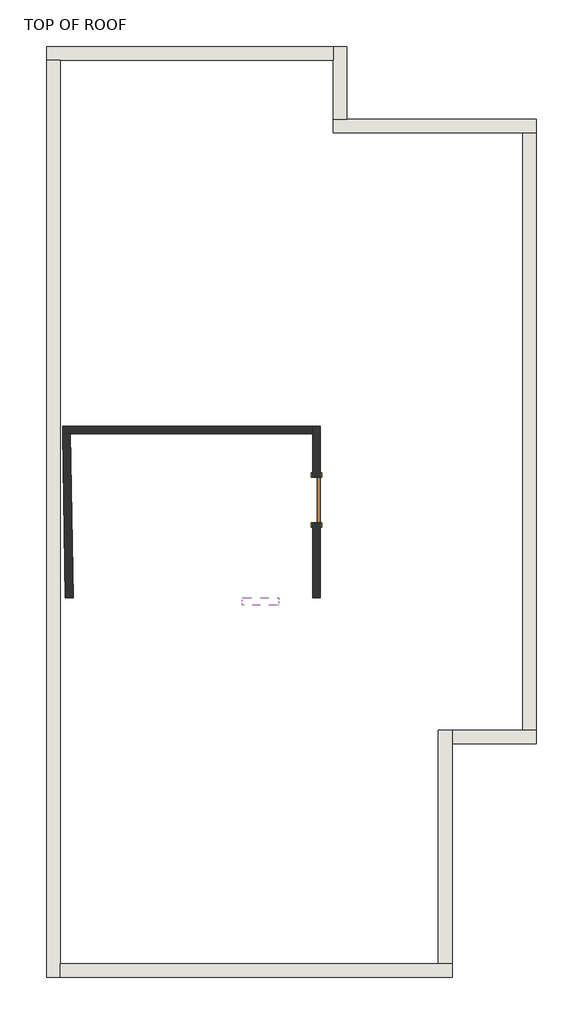
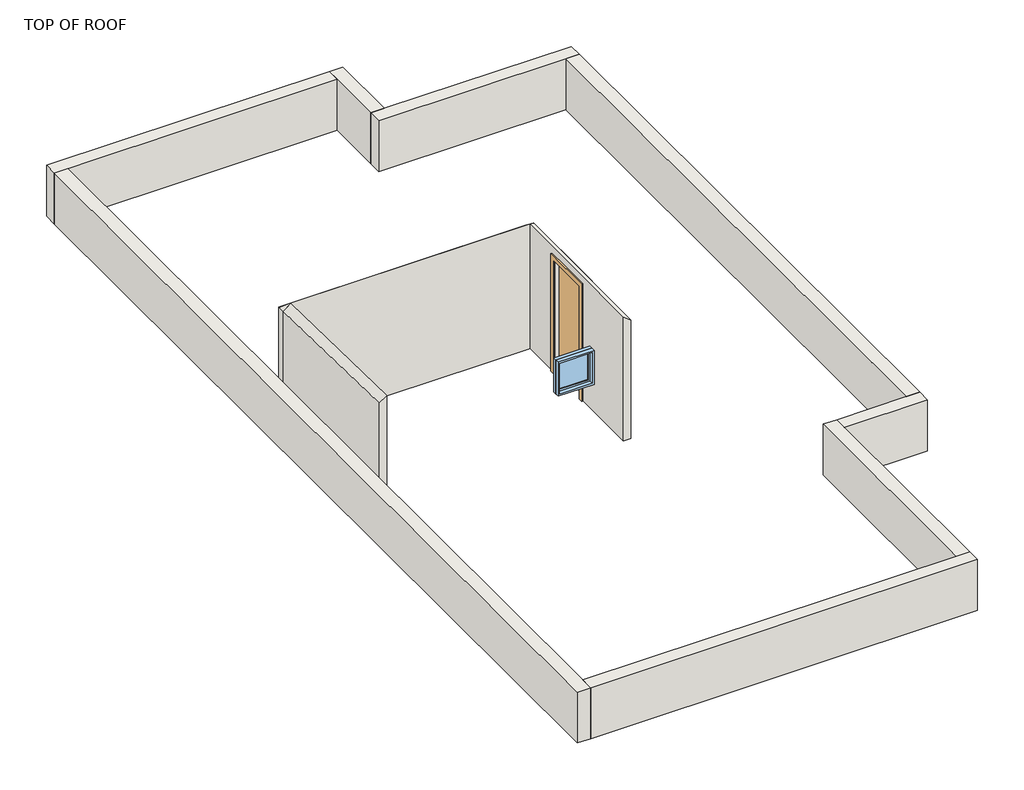
# One storey, incomplete: 11 walls, 1 door, 1 window.
"""IFC4 building model written with IfcOpenShell, lengths in millimetres."""

from ifc_helpers import new_model, si_unit, frame, origin, place, context, project, spatial, polyline, outline, extrude, faceted_brep, transform, mapped, element, save
from components import door_1fe7f57d, window_d757e824

model = new_model("IFC4")

# Units and contexts
model_context = context("Model", 3, world=origin())
ifc_project = project(units=[si_unit("LENGTHUNIT", "METRE", prefix="MILLI")], contexts=[model_context])

# Site, building, storey
site = spatial("IfcSite", under=ifc_project)
building = spatial("IfcBuilding", under=site)
storey = spatial("IfcBuildingStorey", under=building, Name="TOP OF ROOF", Elevation=6400.8)

# Door
placement = place(None, origin())
door_shape = door_1fe7f57d(model_context)
element("IfcDoor", 1, ObjectType="Single-Flush : 30\" x 80\"", at=placement, inside=storey, context=model_context, shape_type="MappedRepresentation", body=[
    mapped(door_shape, transform((-2786.5718918, 4228.995896, 6400.8), x_axis=(0.0, -1.0, 0.0), y_axis=(1.0, 0.0, 0.0), z_axis=(0.0, 0.0, 1.0))),
])

# Walls
element("IfcWall", 2, ObjectType="INNER WALL 5\"", at=placement, inside=storey, context=model_context, shape_type="Brep", body=[
    faceted_brep([(-2723.0718918, 2590.695896, 6400.8), (-2723.0718918, 3847.995896, 6400.8), (-2723.0718918, 3847.995896, 8432.8), (-2723.0718918, 4609.995896, 8432.8), (-2723.0718918, 4609.995896, 6400.8), (-2723.0718918, 5460.895896, 6400.8), (-2723.0718918, 5460.895896, 8534.4), (-2723.0718918, 5449.6118978, 8534.4), (-2723.0718918, 2590.695896, 8534.4), (-2850.0718918, 3847.995896, 8432.8), (-2850.0718918, 3847.995896, 6400.8), (-2850.0718918, 2590.695896, 6400.8), (-2850.0718918, 2590.695896, 8629.65), (-2850.0718918, 5333.895896, 8629.65), (-2850.0718918, 5337.666737, 8629.65), (-2850.0718918, 5449.6118978, 8534.4), (-2850.0718918, 5460.895896, 8534.4), (-2850.0718918, 5460.895896, 6400.8), (-2850.0718918, 5333.895896, 6400.8), (-2850.0718918, 4609.995896, 6400.8), (-2850.0718918, 4609.995896, 8432.8)], [[[0, 1, 2, 3, 4, 5, 6, 7, 8]], [[9, 10, 11, 12, 13, 14, 15, 16, 17, 18, 19, 20]], [[11, 10, 1, 0]], [[19, 18, 17, 5, 4]], [[0, 8, 12, 11]], [[6, 5, 17, 16]], [[8, 7, 14, 13, 12]], [[7, 6, 16, 15]], [[15, 14, 7]], [[2, 1, 10, 9]], [[3, 2, 9, 20]], [[4, 3, 20, 19]]]),
])
element("IfcWall", 3, ObjectType="INNER WALL 5\"", at=placement, inside=storey, context=model_context, shape_type="Brep", body=[
    faceted_brep([(-2850.0718918, 5460.895896, 6400.8), (-7041.0718918, 5460.895896, 6400.8), (-7041.0718918, 5460.895896, 8534.4), (-2850.0718918, 5460.895896, 8534.4), (-2850.0718918, 5333.895896, 6400.8), (-2850.0718918, 5333.895896, 8629.65), (-2854.3498507, 5333.895896, 8632.8584692), (-6907.6225354, 5333.895896, 8632.8584692), (-6911.9011088, 5333.895896, 8629.65), (-7038.9193494, 5333.895896, 8534.4), (-7038.9193494, 5333.895896, 6400.8), (-6911.9011088, 5333.895896, 6400.8), (-2850.0718918, 5449.6118978, 8534.4), (-2850.0718918, 5337.666737, 8629.65), (-7040.8806375, 5449.6118978, 8534.4)], [[[0, 1, 2, 3]], [[4, 5, 6, 7, 8, 9, 10, 11]], [[1, 0, 4, 11, 10]], [[0, 3, 12, 13, 5, 4]], [[2, 1, 10, 9, 14]], [[3, 2, 14, 12]], [[14, 9, 8, 7]], [[7, 6, 13, 12, 14]], [[6, 5, 13]]]),
])
element("IfcWall", 4, ObjectType="INNER WALL 5\"", at=placement, inside=storey, context=model_context, shape_type="Brep", body=[
    faceted_brep([(-7038.9193494, 5333.895896, 6400.8), (-6992.4244341, 2590.695896, 6400.8), (-6992.4244341, 2590.695896, 8534.4), (-7038.9193494, 5333.895896, 8534.4), (-6911.9011088, 5333.895896, 6400.8), (-6911.9011088, 5333.895896, 8629.65), (-6865.4061936, 2590.695896, 8629.65), (-6865.4061936, 2590.695896, 6400.8)], [[[0, 1, 2, 3]], [[4, 5, 6, 7]], [[1, 0, 4, 7]], [[2, 1, 7, 6]], [[0, 3, 5, 4]], [[3, 2, 6, 5]]]),
])
element("IfcWall", 5, ObjectType="OUTER WALL 9\"", at=placement, inside=storey, context=model_context, shape_type="Brep", body=[
    faceted_brep([(895.326752, 10603.9133697, 6400.8), (-2279.673248, 10603.9133697, 6400.8), (-2508.273248, 10603.9133697, 6400.8), (-2508.273248, 10603.9133697, 7315.2), (-2279.673248, 10603.9133697, 7315.2), (895.326752, 10603.9133697, 7315.2), (895.326752, 10375.3133697, 6400.8), (895.326752, 10375.3133697, 7315.2), (666.726752, 10375.3133697, 7315.2), (-2508.273248, 10375.3133697, 7315.2), (-2508.273248, 10375.3133697, 6400.8), (666.726752, 10375.3133697, 6400.8)], [[[0, 1, 2, 3, 4, 5]], [[6, 7, 8, 9, 10, 11]], [[2, 1, 0, 6, 11, 10]], [[5, 4, 3, 9, 8, 7]], [[3, 2, 10, 9]], [[0, 5, 7, 6]]]),
])
element("IfcWall", 6, ObjectType="OUTER WALL 9\"", at=placement, inside=storey, context=model_context, shape_type="Brep", body=[
    faceted_brep([(-2279.673248, 10603.9133697, 6400.8), (-2279.673248, 11823.1133697, 6400.8), (-2279.673248, 11823.1133697, 7315.2), (-2279.673248, 10603.9133697, 7315.2), (-2508.273248, 10603.9133697, 6400.8), (-2508.273248, 10603.9133697, 7315.2), (-2508.273248, 11594.5133697, 7315.2), (-2508.273248, 11823.1133697, 7315.2), (-2508.273248, 11823.1133697, 6400.8), (-2508.273248, 11594.5133697, 6400.8)], [[[0, 1, 2, 3]], [[4, 5, 6, 7, 8, 9]], [[1, 0, 4, 9, 8]], [[3, 2, 7, 6, 5]], [[0, 3, 5, 4]], [[2, 1, 8, 7]]]),
])
element("IfcWall", 7, ObjectType="OUTER WALL 9\"", at=placement, inside=storey, context=model_context, shape_type="Brep", body=[
    faceted_brep([(-2508.273248, 11823.1133697, 6400.8), (-7308.873248, 11823.1133697, 6400.8), (-7308.873248, 11823.1133697, 7315.2), (-2508.273248, 11823.1133697, 7315.2), (-2508.273248, 11594.5133697, 6400.8), (-2508.273248, 11594.5133697, 7315.2), (-7080.273248, 11594.5133697, 7315.2), (-7308.873248, 11594.5133697, 7315.2), (-7308.873248, 11594.5133697, 6400.8), (-7080.273248, 11594.5133697, 6400.8)], [[[0, 1, 2, 3]], [[4, 5, 6, 7, 8, 9]], [[1, 0, 4, 9, 8]], [[3, 2, 7, 6, 5]], [[0, 3, 5, 4]], [[2, 1, 8, 7]]]),
])
element("IfcWall", 8, ObjectType="OUTER WALL 9\"", at=placement, inside=storey, context=model_context, shape_type="Brep", body=[
    faceted_brep([(-7308.873248, 11594.5133697, 6400.8), (-7308.873248, -3772.4866303, 6400.8), (-7308.873248, -3772.4866303, 7315.2), (-7308.873248, 11594.5133697, 7315.2), (-7080.273248, 11594.5133697, 6400.8), (-7080.273248, 11594.5133697, 7315.2), (-7080.273248, -3543.8866303, 7315.2), (-7080.273248, -3772.4866303, 7315.2), (-7080.273248, -3772.4866303, 6400.8), (-7080.273248, -3543.8866303, 6400.8)], [[[0, 1, 2, 3]], [[4, 5, 6, 7, 8, 9]], [[1, 0, 4, 9, 8]], [[3, 2, 7, 6, 5]], [[0, 3, 5, 4]], [[2, 1, 8, 7]]]),
])
element("IfcWall", 9, ObjectType="OUTER WALL 9\"", at=placement, inside=storey, context=model_context, shape_type="Brep", body=[
    faceted_brep([(-7080.273248, -3772.4866303, 6400.8), (-514.373248, -3772.4866303, 6400.8), (-514.373248, -3772.4866303, 7315.2), (-7080.273248, -3772.4866303, 7315.2), (-7080.273248, -3543.8866303, 6400.8), (-7080.273248, -3543.8866303, 7315.2), (-742.973248, -3543.8866303, 7315.2), (-514.373248, -3543.8866303, 7315.2), (-514.373248, -3543.8866303, 6400.8), (-742.973248, -3543.8866303, 6400.8)], [[[0, 1, 2, 3]], [[4, 5, 6, 7, 8, 9]], [[1, 0, 4, 9, 8]], [[3, 2, 7, 6, 5]], [[0, 3, 5, 4]], [[2, 1, 8, 7]]]),
])
element("IfcWall", 10, ObjectType="OUTER WALL 9\"", at=placement, inside=storey, context=model_context, shape_type="Brep", body=[
    faceted_brep([(-514.373248, -3543.8866303, 6400.8), (-514.373248, 139.1133697, 6400.8), (-514.373248, 367.7133697, 6400.8), (-514.373248, 367.7133697, 7315.2), (-514.373248, 139.1133697, 7315.2), (-514.373248, -3543.8866303, 7315.2), (-742.973248, -3543.8866303, 6400.8), (-742.973248, -3543.8866303, 7315.2), (-742.973248, 367.7133697, 7315.2), (-742.973248, 367.7133697, 6400.8)], [[[0, 1, 2, 3, 4, 5]], [[6, 7, 8, 9]], [[2, 1, 0, 6, 9]], [[5, 4, 3, 8, 7]], [[0, 5, 7, 6]], [[3, 2, 9, 8]]]),
])
element("IfcWall", 11, ObjectType="OUTER WALL 9\"", at=placement, inside=storey, context=model_context, shape_type="Brep", body=[
    faceted_brep([(-514.373248, 139.1133697, 6400.8), (895.326752, 139.1133697, 6400.8), (895.326752, 139.1133697, 7315.2), (-514.373248, 139.1133697, 7315.2), (-514.373248, 367.7133697, 6400.8), (-514.373248, 367.7133697, 7315.2), (666.726752, 367.7133697, 7315.2), (895.326752, 367.7133697, 7315.2), (895.326752, 367.7133697, 6400.8), (666.726752, 367.7133697, 6400.8)], [[[0, 1, 2, 3]], [[4, 5, 6, 7, 8, 9]], [[1, 0, 4, 9, 8]], [[3, 2, 7, 6, 5]], [[0, 3, 5, 4]], [[2, 1, 8, 7]]]),
])
element("IfcWall", 12, ObjectType="OUTER WALL 9\"", at=placement, inside=storey, context=model_context, shape_type="SweptSolid", body=[
    extrude(outline(polyline([(895.326752, 10375.3133697), (895.326752, 367.7133697), (666.726752, 367.7133697), (666.726752, 10375.3133697), (895.326752, 10375.3133697)])), frame((0.0, 0.0, 6400.8), z_axis=(0.0, 0.0, 1.0), x_axis=(1.0, 0.0, 0.0)), (0.0, 0.0, 1.0), 914.4),
])

# Window
window_shape = window_d757e824(model_context)
element("IfcWindow", 13, ObjectType="Fixed : 24\" x 24\"", at=placement, inside=storey, context=model_context, shape_type="MappedRepresentation", body=[
    mapped(window_shape, transform((-3688.2718918, 2527.195896, 6784.2359609), x_axis=(1.0, 0.0, 0.0), y_axis=(0.0, 1.0, 0.0), z_axis=(0.0, 0.0, 1.0))),
])

save(model, "model.ifc")

# Revit data of these elements
# Type "Single-Flush : 30\" x 80\""
#   Type Mark = "5"
#   Construction Type Id = "MDOOR"
#   Assembly Code = "C1020"
#   Analytic Construction = "Metal"
#   Thickness = 0' - 2"
#   Heat Transfer Coefficient (U) = 0.651978 BTU/(h·ft²·°F)
#   Height = 6' - 8"
#   Trim Projection Ext = 0' - 1"
#   Trim Projection Int = 0' - 1"
#   Trim Width = 0' - 3"
#   Width = 2' - 6"
#   Define Thermal Properties by = 1
#   Define Thermal Properties by = 1
#   Door Material = Door - Panel
#   Frame Material = Door - Frame
#   Visual Light Transmittance = 0
#   Solar Heat Gain Coefficient = 0
#   Function = (empty or 0)
#   Wall Closure = (empty or 0)
# Type "INNER WALL 5\""
#   Assembly Code = "B2010"
#   Layers, outside or top first: 0' - 5" "IVORY WHITE COLOUR" (function 1)
# Type "OUTER WALL 9\""
#   Assembly Code = "B2010"
#   Layers, outside or top first: 0' - 9" "IVORY WHITE COLOUR" (function 1)
# Type "Fixed : 24\" x 24\""
#   Type Mark = "3"
#   Construction Type Id = "GSP4R"
#   Assembly Code = "B2020100"
#   Analytic Construction = "1/8 in Pilkington single glazing"
#   Visual Light Transmittance = 0.9
#   Solar Heat Gain Coefficient = 0.78
#   Heat Transfer Coefficient (U) = 0.6496 BTU/(h·ft²·°F)
#   Height = 2' - 0"
#   Default Sill Height = 3' - 0"
#   Width = 2' - 0"
#   Window Inset = 0' - 0 3/4"
#   Define Thermal Properties by = 1
#   Define Thermal Properties by = 1
#   Glass Pane Material = Glass
#   Sash Material = Sash
#   Wall Closure = (empty or 0)
# Element 1 (IfcDoor, "Single-Flush : 30\" x 80\"")
#   Phase Created = New Construction
#   Materials on its faces: "Door - Frame", "Door - Panel"
# Elements 2, 3, 4 (IfcWall, "INNER WALL 5\"")
#   Top Offset = 0' - 0"
#   Base Offset = 0' - 0"
#   Unconnected Height = 7' - 0"
#   wall height = 7' - 0"
#   Phase Created = New Construction
#   Base Constraint = TOP OF ROOF
#   Materials on its faces: "IVORY WHITE COLOUR"
# Elements 5, 6, 7, 8, 9, 10, 11, 12 (IfcWall, "OUTER WALL 9\"")
#   Top Offset = 0' - 0"
#   Base Offset = 0' - 0"
#   Unconnected Height = 3' - 0"
#   wall height = 3' - 0"
#   Phase Created = New Construction
#   Base Constraint = TOP OF ROOF
#   Materials on its faces: "IVORY WHITE COLOUR"
# Element 13 (IfcWindow, "Fixed : 24\" x 24\"")
#   Mark = "11"
#   Phase Created = New Construction
#   Materials on its faces: "Sash", "Glass"
# Materials
#   "Door - Panel": class "Wood", colour RGB 210 159 95, transparency 0, Cost = 0
#   "Door - Frame": colour RGB 118 70 51, transparency 0, Cost = 0
#   "IVORY WHITE COLOUR": class "Generic", colour RGB 120 120 120, transparency 0, Cost = 0
#   "Glass": class "Glass", colour RGB 0 128 192, transparency 0.75, Description = "Soda Lime Glass", Cost = 0
#   "Sash": class "Wood", colour RGB 224 178 126, transparency 0, Cost = 0
